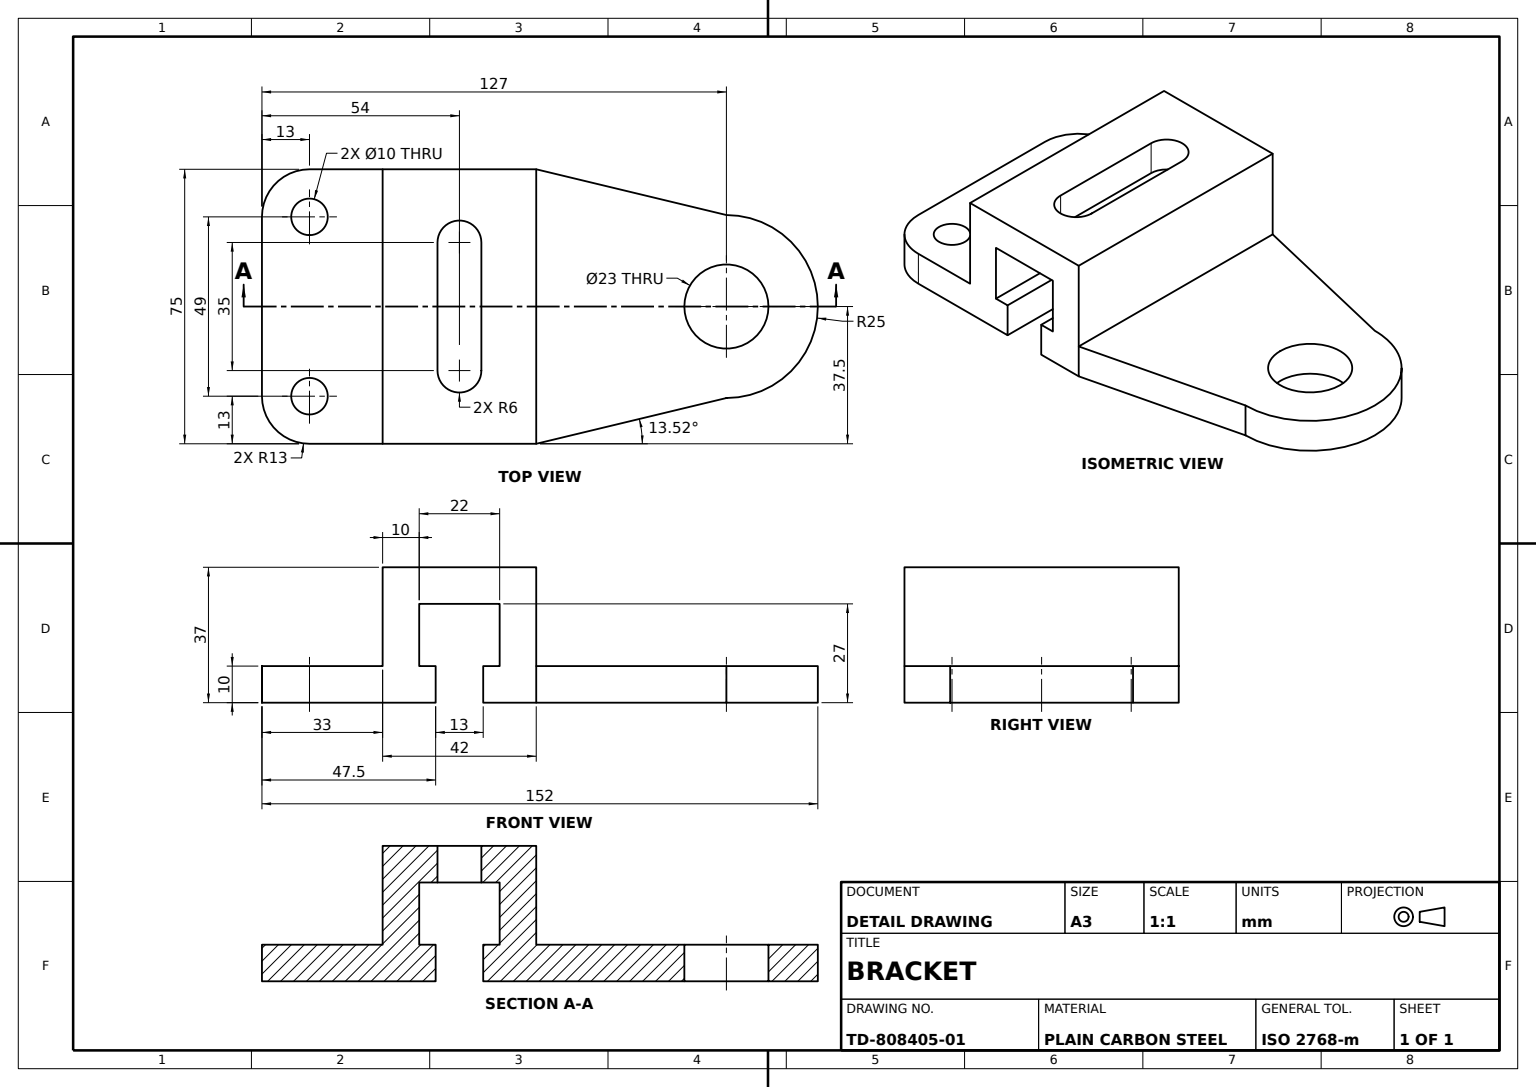
from build123d import *

# Parameters (mm, degrees)
BASE_BODY_DEPTH              = 37.5
UPPER_FLANGE_DEPTH           = 75
FLANGE_CORNER_FILLET_R13_A_R = 13
FLANGE_CORNER_FILLET_R13_B_R = 13
MOUNTING_HOLES_SKETCH_R      = 5
MOUNTING_HOLES_2X_10_DEPTH   = 75
SLOT_6MM_DEPTH               = 75
HANGER_PLATE_DEPTH           = 75
TAPER_CUT_DEPTH              = 75
EYE_BOSS_SKETCH_R            = 25
EYE_BOSS_DEPTH               = 10
EYE_HOLE_SKETCH_R            = 11.5
EYE_HOLE_23_DEPTH            = 10


with BuildPart() as part:
    # Base Profile Sketch → Base Body (new, symmetric)
    with BuildSketch(Plane.XY):
        Polygon((0, 11), (0, 21), (-27, 21), (-27, -21), (0, -21), (0, -11), (-17, -11), (-17, 11), align=None)
    extrude(amount=BASE_BODY_DEPTH, both=True)

    # Upper Flange Sketch → Upper Flange (add)
    with BuildSketch(Plane.XY.offset(37.5)):
        Polygon((0, 21), (0, 54), (10, 54), (10, 21), (10, 6.5), (0, 6.5), align=None)
    extrude(amount=-UPPER_FLANGE_DEPTH)

    # Flange Corner Fillet R13 A
    flange_corner_fillet_r13_a_edges = [part.edges().sort_by_distance(p)[0] for p in [
        (5, 54, 37.5),
    ]]
    fillet(flange_corner_fillet_r13_a_edges, radius=FLANGE_CORNER_FILLET_R13_A_R)

    # Flange Corner Fillet R13 B
    flange_corner_fillet_r13_b_edges = [part.edges().sort_by_distance(p)[0] for p in [
        (5, 54, -37.5),
    ]]
    fillet(flange_corner_fillet_r13_b_edges, radius=FLANGE_CORNER_FILLET_R13_B_R)

    # Mounting Holes Sketch → Mounting Holes 2xØ10 (cut)
    with BuildSketch(Plane.ZY):
        with Locations((24.5, 41)):
            Circle(MOUNTING_HOLES_SKETCH_R)
        with Locations((-24.5, 41)):
            Circle(MOUNTING_HOLES_SKETCH_R)
    extrude(amount=-MOUNTING_HOLES_2X_10_DEPTH, mode=Mode.SUBTRACT)

    # Slot Sketch → Slot 6mm (cut)
    with BuildSketch(Plane.ZY.offset(27)):
        with BuildLine():
            Line((-17.5, 6), (17.5, 6))
            ThreePointArc((17.5, 6), (23.5, 0), (17.5, -6))
            Line((17.5, -6), (-17.5, -6))
            ThreePointArc((-17.5, -6), (-23.5, 0), (-17.5, 6))
        make_face()
    extrude(amount=-SLOT_6MM_DEPTH, mode=Mode.SUBTRACT)

    # Hanger Plate Sketch → Hanger Plate (add)
    with BuildSketch(Plane.XY.offset(37.5)):
        Polygon((0, -6.5), (0, -21), (0, -73), (10, -73), (10, -21), (10, -6.5), align=None)
    extrude(amount=-HANGER_PLATE_DEPTH)

    # Taper Cut Sketch → Taper Cut (cut)
    with BuildSketch(Plane.ZY):
        Polygon((37.5, -73), (37.5, -21), (25, -73), align=None)
        Polygon((-25, -73), (-37.5, -21), (-37.5, -73), align=None)
    extrude(amount=-TAPER_CUT_DEPTH, mode=Mode.SUBTRACT)

    # Eye Boss Sketch → Eye Boss (add)
    with BuildSketch(Plane.ZY):
        with Locations((0, -73)):
            Circle(EYE_BOSS_SKETCH_R)
    extrude(amount=-EYE_BOSS_DEPTH)

    # Eye Hole Sketch → Eye Hole Ø23 (cut)
    with BuildSketch(Plane.ZY):
        with Locations(Location((0, -73, 0), (0, 0, 270))):
            Circle(EYE_HOLE_SKETCH_R)
    extrude(amount=-EYE_HOLE_23_DEPTH, mode=Mode.SUBTRACT)


solid = part.part
